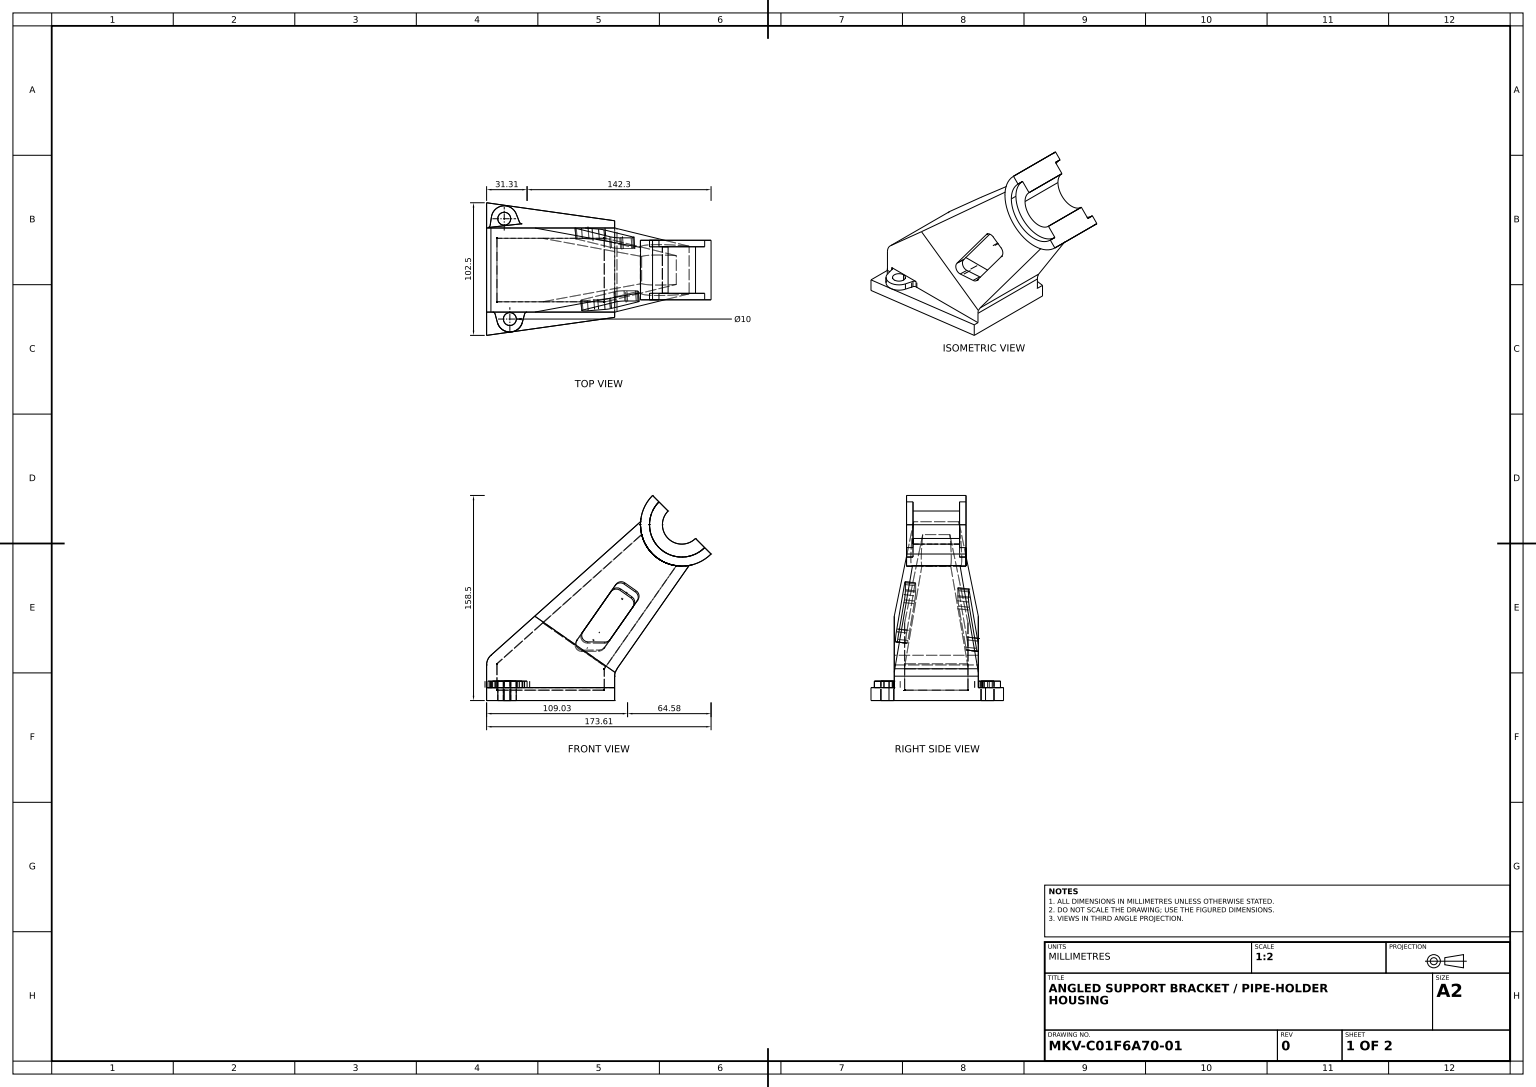
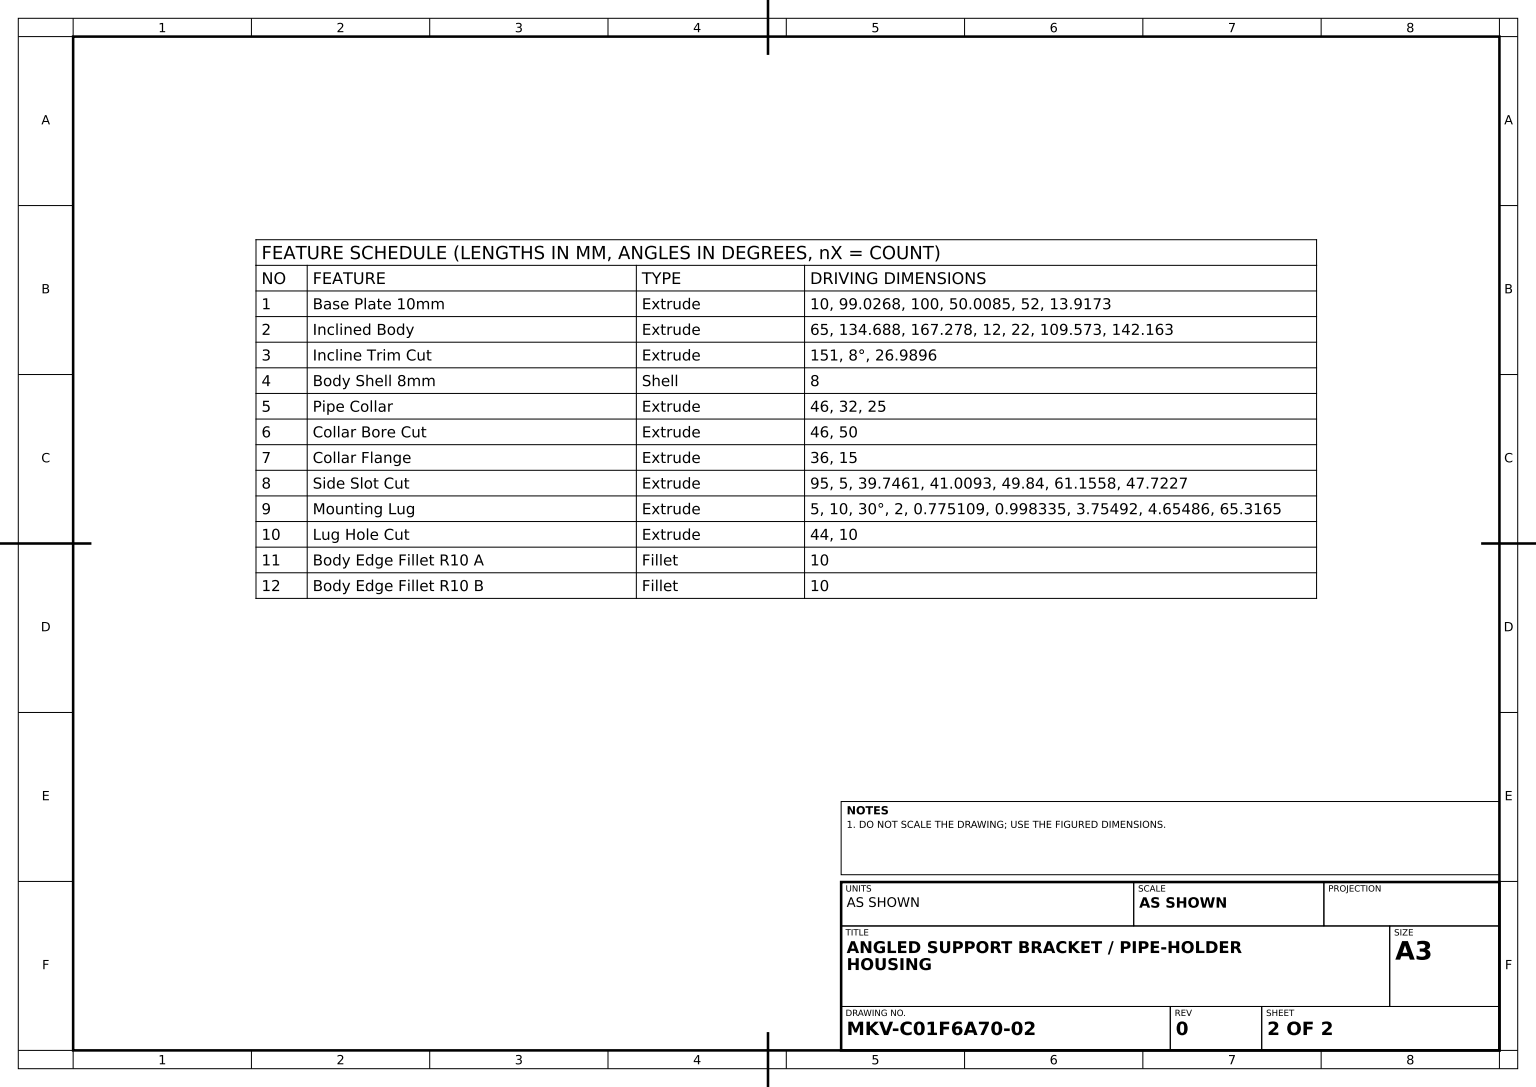
from build123d import *

# Parameters (mm, degrees)
BASE_PLATE_10MM_DEPTH    = 10
INCLINED_BODY_DEPTH      = 32.5
INCLINE_TRIM_CUT_DEPTH   = 151
BODY_SHELL_8MM_T         = -8
PIPE_COLLAR_DEPTH        = 23
COLLAR_BORE_SKETCH_R     = 25
COLLAR_BORE_CUT_DEPTH    = 46
COLLAR_FLANGE_DEPTH      = 18
SIDE_SLOT_CUT_DEPTH      = 95
MOUNTING_LUG_DEPTH       = 5
LUG_HOLE_SKETCH_R        = 5
LUG_HOLE_CUT_DEPTH       = 44
BODY_EDGE_FILLET_R10_A_R = 10
BODY_EDGE_FILLET_R10_B_R = 10


with BuildPart() as part:
    # Base Plate Sketch → Base Plate 10mm (new body)
    with BuildSketch(Plane(origin=(0, 0, 0), x_dir=(1, 0, 0), z_dir=(0, 1, 0))):
        Polygon((0, 0), (0, 52), (99.026806874, 38.082689904), (99.026806874, -36.582689904), (0, -50.5), align=None)
    extrude(amount=BASE_PLATE_10MM_DEPTH)

    # Inclined Body Sketch → Inclined Body (add, symmetric)
    with BuildSketch(Plane.XY):
        Polygon((0, 10), (0, 32), (134.688366927, 152.162572436), (167.277586184, 119.573353179), (99.026806874, 22), (99.026806874, 10), align=None)
    extrude(amount=INCLINED_BODY_DEPTH, both=True)

    # Incline Trim Sketch → Incline Trim Cut (cut)
    with BuildSketch(Plane(origin=(56.160363076, -39.283148743, 0), x_dir=(0, 0, -1), z_dir=(0.8194313825543525, -0.5731772930647745, 0))):
        Polygon((32.5, 74.787407521), (5.510372788, 266.828583807), (32.5, 266.828583807), (32.5, 193.861872152), align=None)
        Polygon((-32.5, 74.787407521), (-5.510372788, 266.828583807), (-32.5, 266.828583807), (-32.5, 193.861872152), align=None)
    extrude(amount=-INCLINE_TRIM_CUT_DEPTH, mode=Mode.SUBTRACT)

    # Body Shell 8mm
    body_shell_8mm_openings = [part.faces().sort_by_distance(p)[0] for p in [
        (151.184475908, 135.666463456, 0),
    ]]
    offset(amount=BODY_SHELL_8MM_T, openings=body_shell_8mm_openings, kind=Kind.INTERSECTION)

    # Pipe Collar Sketch → Pipe Collar (add, symmetric)
    with BuildSketch(Plane.XY):
        with BuildLine():
            Line((168.660646085, 118.190293278), (173.610393554, 113.24054581))
            ThreePointArc((173.610393554, 113.24054581), (128.355559558, 113.24054581), (128.355559558, 158.495379806))
            Line((128.355559558, 158.495379806), (133.305307026, 153.545632337))
            ThreePointArc((133.305307026, 153.545632337), (133.305307026, 118.190293278), (168.660646085, 118.190293278))
        make_face()
    extrude(amount=PIPE_COLLAR_DEPTH, both=True)

    # Collar Bore Sketch → Collar Bore Cut (cut)
    with BuildSketch(Plane.XY.offset(23)):
        with Locations((150.982976556, 135.867962808)):
            Circle(COLLAR_BORE_SKETCH_R)
    extrude(amount=-COLLAR_BORE_CUT_DEPTH, mode=Mode.SUBTRACT)

    # Collar Flange Sketch → Collar Flange (add, symmetric)
    with BuildSketch(Plane.XY):
        with BuildLine():
            Line((133.305307026, 153.545632337), (140.376374838, 146.474564526))
            ThreePointArc((140.376374838, 146.474564526), (140.376374838, 125.26136109), (161.589578273, 125.26136109))
            Line((161.589578273, 125.26136109), (168.660646085, 118.190293278))
            ThreePointArc((168.660646085, 118.190293278), (133.305307026, 118.190293278), (133.305307026, 153.545632337))
        make_face()
    extrude(amount=COLLAR_FLANGE_DEPTH, both=True)

    # Side Slot Sketch → Side Slot Cut (cut)
    with BuildSketch(Plane(origin=(3.397609111, 4.857323493, 42.177604188), x_dir=(0.9968132270848588, -0.009126376589251743, -0.07924707918290198), z_dir=(0.07977086127571884, 0.11404280653407992, 0.9902680687415709))):
        with BuildLine():
            Line((92.581603623, 43.613463299), (113.99131411, 74.522227016))
            ThreePointArc((113.99131411, 74.522227016), (114.800629853, 78.262503606), (112.728127564, 81.479551196))
            Line((112.728127564, 81.479551196), (103.897429804, 87.596349789))
            ThreePointArc((103.897429804, 87.596349789), (100.157153215, 88.405665533), (96.940105624, 86.333163243))
            Line((96.940105624, 86.333163243), (71.29344512, 49.307600933))
            ThreePointArc((71.29344512, 49.307600933), (70.974516355, 44.140547642), (75.403700483, 41.460532116))
            Line((75.403700483, 41.460532116), (88.47134826, 41.460532116))
            ThreePointArc((88.47134826, 41.460532116), (90.791332734, 42.031347987), (92.581603623, 43.613463299))
        make_face()
    extrude(amount=-SIDE_SLOT_CUT_DEPTH, mode=Mode.SUBTRACT)

    # Mounting Lug Sketch → Mounting Lug (add)
    with BuildSketch(Plane(origin=(0, 10, 0), x_dir=(1, 0, 0), z_dir=(0, 1, 0))):
        with BuildLine():
            ThreePointArc((3.754917352, 41.138806093), (12.526564043, 49.582407535), (22.952725963, 43.29501232))
            Line((22.952725963, 43.29501232), (25.401555204, 37.04901044))
            ThreePointArc((25.401555204, 37.04901044), (26.230743087, 36.066350412), (27.486787588, 35.791531397))
            Line((27.486787588, 35.791531397), (0.998335406, 32.816474884))
            ThreePointArc((0.998335406, 32.816474884), (2.162121722, 33.363077745), (2.752664744, 34.505195172))
            Line((2.752664744, 34.505195172), (3.754917352, 41.138806093))
        make_face()
        with BuildLine():
            Line((31.309858058, -32.5), (4.654857397, -32.5))
            ThreePointArc((4.654857397, -32.5), (5.872380255, -32.913293319), (6.58670905, -33.98236191))
            Line((6.58670905, -33.98236191), (8.323099465, -40.462659161))
            ThreePointArc((8.323099465, -40.462659161), (12.462987997, -46.213327011), (19.374089028, -47.777149356))
            ThreePointArc((19.374089028, -47.777149356), (24.60855832, -45.364025821), (27.641615991, -40.462659161))
            Line((27.641615991, -40.462659161), (29.378006406, -33.98236191))
            ThreePointArc((29.378006406, -33.98236191), (30.0923352, -32.913293319), (31.309858058, -32.5))
        make_face()
    extrude(amount=MOUNTING_LUG_DEPTH)

    # Lug Hole Sketch → Lug Hole Cut (cut)
    with BuildSketch(Plane(origin=(0, 15, 0), x_dir=(1, 0, 0), z_dir=(0, 1, 0))):
        with Locations(Location((13.642698516, 39.64489055, 0), (0, 0, 270))):
            Circle(LUG_HOLE_SKETCH_R)
        with Locations(Location((17.982357728, -37.87446871, 0), (0, 0, 270))):
            Circle(LUG_HOLE_SKETCH_R)
    extrude(amount=-LUG_HOLE_CUT_DEPTH, mode=Mode.SUBTRACT)

    # Body Edge Fillet R10 A
    body_edge_fillet_r10_a_edges = [part.edges().sort_by_distance(p)[0] for p in [
        (0, 32, 0),
    ]]
    fillet(body_edge_fillet_r10_a_edges, radius=BODY_EDGE_FILLET_R10_A_R)

    # Body Edge Fillet R10 B
    body_edge_fillet_r10_b_edges = [part.edges().sort_by_distance(p)[0] for p in [
        (99.026806874, 22, 0),
    ]]
    fillet(body_edge_fillet_r10_b_edges, radius=BODY_EDGE_FILLET_R10_B_R)


solid = part.part
